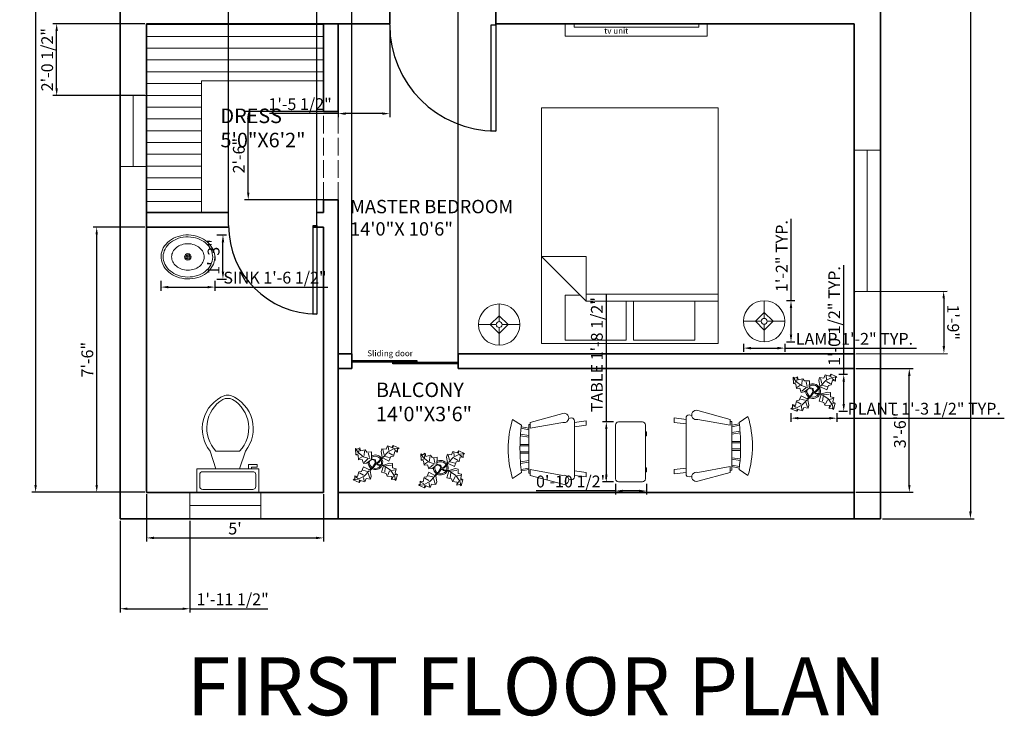
# Model space of a CAD drawing. Units: inches. Extents: x 2170 to 3011, y 1733 to 2338.
# Tile 4 of 5: x 2677 to 3011, y 1737 to 1974. Entities that reach past the tile are written whole.
import ezdxf

# ---------------------------------------------------------------- set-up
doc = ezdxf.new("R2010")
doc.units = ezdxf.units.IN
doc.linetypes.add('ACAD_ISO02W100', pattern=[15, 12, -3])
for name, color, linetype, lineweight in [('A-AREA-IDEN', 4, 'Continuous', 18), ('A-FLOR-CASE', 20, 'Continuous', 20), ('A-FLOR-CASE-PATT', 252, 'Continuous', 13), ('A-FLOR-FIXT', 20, 'Continuous', 18), ('A-WALL', 7, 'Continuous', 35), ('A-WALL-OVHD', 7, 'ACAD_ISO02W100', 18), ('dim', 11, 'Continuous', 18), ('door', 6, 'Continuous', 25), ('furnitures', 20, 'Continuous', 18), ('L-PLNT', 81, 'Continuous', 13), ('text', 4, 'Continuous', 18), ('window', 3, 'Continuous', 20)]:
    doc.layers.add(name, color=color, linetype=linetype, lineweight=lineweight)
doc.styles.get("Standard").update_dxf_attribs({"font": 'arial.ttf'})
doc.dimstyles.new('ISO-25', dxfattribs={"dimtxt": 4, "dimasz": 2.5, "dimexe": 1.25, "dimexo": 0.625, "dimtad": 1, "dimlunit": 3, "dimtxsty": 'Standard', "dimcen": 2.5, "dimadec": 0, "dimazin": 0, "dimtfac": 1, "dimtmove": 0, "dimatfit": 3, "dimfxl": 1, "dimarcsym": 0})

# ---------------------------------------------------------------- blocks, each defined once
blk = doc.blocks.new('*D36')
at = {"layer": 'Defpoints', "color": 0, "transparency": 16777216}
for p in [(2719.6, 2293.31), (2681.96, 1813.31), (2719.6, 1813.31)]:
    blk.add_point(p, dxfattribs=at)
at = {"layer": 'dim', "color": 0, "lineweight": -2, "transparency": 16777216}
for p, q in [((2718.97, 2293.31), (2680.71, 2293.31)), ((2681.96, 2290.81), (2681.96, 1815.81)), ((2718.97, 1813.31), (2680.71, 1813.31))]:
    blk.add_line(p, q, dxfattribs=at)
at = {"layer": 'dim', "color": 0, "transparency": 16777216}
for points in [[(2681.54, 2290.81), (2682.37, 2290.81), (2681.96, 2293.31)], [(2681.54, 1815.81), (2682.37, 1815.81), (2681.96, 1813.31)]]:
    blk.add_solid(points, dxfattribs=at)
at = {"layer": 'dim', "color": 0, "transparency": 16777216, "insert": (2679.29, 2053.31), "char_height": 4, "attachment_point": 5, "rotation": 90}
blk.add_mtext("40'", dxfattribs=at)
blk = doc.blocks.new('*U37')
for p, q in [((-40, 0), (-40, 6)), ((0, 0), (0, 6))]:
    blk.add_line(p, q)
blk.add_lwpolyline([(0, 0), (0, -40), (-1.75, -40), (-1.75, 0)], close=True)
blk.add_arc((0, 0), 40, 180, 270)
blk = doc.blocks.new('Bed - Queen')
for p, q in [((0, -80.00003), (0, 0)), ((0, 0), (59.99999, 0)), ((59.99999, 0), (59.99999, -80.00003)), ((7.99999, -1.2), (28.79998, -1.2)), ((7.99999, -14.4), (7.99999, -1.2)), ((28.79998, -1.2), (28.79998, -14.4)), ((31.19999, -1.2), (51.99999, -1.2)), ((31.19999, -14.4), (31.19999, -1.2)), ((51.99999, -1.2), (51.99999, -16.4)), ((0, -14.4), (44.8, -14.4)), ((59.99999, -29.6), (44.8, -14.4)), ((44.8, -14.4), (44.8, -29.6)), ((51.99999, -16.4), (46.79936, -16.4)), ((44.8, -16.8), (0, -16.8)), ((44.8, -29.6), (59.99999, -29.6)), ((59.99999, -80.00003), (0, -80.00003))]:
    blk.add_line(p, q)
blk = doc.blocks.new('Lamp - Table')
for p, q in [((0, 7), (0, 1)), ((-1, 0), (-7, 0)), ((0, 3), (-3, 0)), ((-3, 0), (0, -3)), ((3, 0), (0, 3)), ((0, -3), (3, 0)), ((1, 0), (7, 0)), ((0, -1), (0, -7))]:
    blk.add_line(p, q)
for radius in [7, 1]:
    blk.add_circle((0, 0), radius)
blk = doc.blocks.new('Plant - Rubber or Philodendron')
for p, q in [((-16.2005, 11.4774), (-13.9899, 8.1064)), ((-16.2005, 11.4774), (-14.8639, 10.7964)), ((-16.0159, 6.3329), (-16.2005, 11.4774)), ((-14.8639, 10.7964), (-12.6195, 11.8975)), ((-13.9899, 8.1064), (-9.5434, 4.7185)), ((-13.3174, 8.325), (-13.0735, 11.0065)), ((-12.6195, 11.8975), (-12.1909, 9.4345)), ((-12.1909, 9.4345), (-8.3829, 10.3)), ((-8.8369, 9.409), (-9.0894, 5.6095)), ((-8.3829, 10.3), (-7.0549, 8.501)), ((-7.0549, 8.501), (-3.0284, 8.6941)), ((-3.0284, 8.6941), (-3.0709, 3.1041)), ((4.6914, 8.8812), (5.3859, 11.2828)), ((4.6914, 8.8812), (5.5014, 4.4831)), ((5.3859, 11.2828), (8.8871, 10.7908)), ((5.9878, 10.4842), (7.1971, 6.3869)), ((10.3916, 8.7942), (6.2847, 4.4028)), ((8.8871, 10.7908), (9.9809, 13.4933)), ((9.9809, 13.4933), (13.3837, 12.301)), ((15.3859, 11.3055), (10.3916, 8.7942)), ((10.5828, 12.6946), (10.8893, 9.7953)), ((13.3837, 12.301), (14.68, 13.9039)), ((14.5816, 13.2037), (14.3848, 11.8033)), ((14.68, 13.9039), (19.3848, 11.8146)), ((15.7909, 9.1065), (14.8995, 5.3044)), ((15.2875, 10.6053), (17.5907, 9.2105)), ((19.3848, 11.8146), (15.3859, 11.3055)), ((18.1925, 8.4119), (15.7909, 9.1065)), ((19.3848, 11.8146), (18.1868, 10.9119)), ((18.1868, 10.9119), (18.1925, 8.4119)), ((-14.0069, 5.8704), (-16.0159, 6.3329)), ((-15.3434, 6.5514), (-13.9984, 6.9884)), ((-13.5868, 2.2894), (-14.0069, 5.8704)), ((-10.6784, 2.491), (-13.5868, 2.2894)), ((-13.1329, 3.1804), (-10.6614, 4.727)), ((-9.5858, -0.8715), (-10.6784, 2.491)), ((-9.5434, 4.7185), (-4.1917, 2.9888)), ((-9.1318, 0.0195), (-5.9793, 2.9025)), ((-7.1228, -0.443), (-3.5248, 2.2131)), ((-4.8529, 4.012), (-5.7184, 7.82)), ((-3.5248, 2.2131), (-3.3011, 2.4355)), ((-3.3011, 2.4355), (-0.5306, 1.7947)), ((-3.0709, 3.1041), (0.0797, 2.3163)), ((-0.5306, 1.7947), (-0.2255, -0.5527)), ((-0.5306, 1.7947), (-0.5306, 1.7947)), ((0.0797, 2.3163), (0.4866, -0.031)), ((0.4866, -0.031), (2.1141, 0.2298)), ((2.1141, 0.2298), (5.4346, 3.9146)), ((6.1032, 3.6844), (2.8262, -0.031)), ((5.4346, 3.9146), (5.5014, 4.4831)), ((11.1089, 1.1958), (6.1032, 3.6844)), ((7.7005, 4.8881), (11.5025, 3.9967)), ((14.2977, 6.1031), (10.9934, 7.9956)), ((12.7005, 4.8994), (11.1089, 1.1958)), ((14.8995, 5.3044), (12.7005, 4.8994)), ((-14.4141, -11.4699), (-13.5228, -7.6679)), ((-13.5228, -7.6679), (-11.3237, -7.2629)), ((-11.3237, -7.2629), (-9.7321, -3.5593)), ((-6.3237, -7.2516), (-10.1257, -6.3602)), ((-9.7321, -3.5593), (-4.7264, -6.0479)), ((-7.1228, -0.443), (-9.5858, -0.8715)), ((-9.0148, -11.1577), (-4.9047, -6.8122)), ((-2.019, -3.6148), (-4.7264, -6.0479)), ((-4.1246, -6.8466), (-4.0579, -6.2781)), ((-3.3146, -11.2447), (-4.1246, -6.8466)), ((-4.0579, -6.2781), (-0.9375, -3.1608)), ((-2.019, -3.6148), (-0.2255, -0.5527)), ((-0.9375, -3.1608), (0.5883, -0.8135)), ((0.5883, -0.8135), (2.2447, -2.0916)), ((2.8262, -0.031), (1.3003, -0.5527)), ((1.3003, -0.5527), (2.4193, -1.4655)), ((2.2447, -2.0916), (6.7108, -2.6626)), ((2.4193, -1.4655), (6.895, -2.1175)), ((4.943, -7.9659), (6.7108, -2.6626)), ((8.8321, -9.0266), (4.943, -7.9659)), ((11.6605, -0.5413), (6.895, -2.1175)), ((12.3677, -6.1981), (7.219, -2.6772)), ((8.125, -4.0768), (7.7715, -7.9659)), ((8.3544, -2.7453), (13.1973, -2.1704)), ((10.2463, -10.4408), (11.6605, -6.9053)), ((11.6605, -0.5413), (14.1354, -0.8948)), ((15.5496, -10.7943), (12.3677, -6.1981)), ((16.2567, -5.8446), (13.4283, -6.5517)), ((14.1354, -0.8948), (14.1354, -4.4304)), ((14.1354, -4.4304), (16.9638, -5.1375)), ((16.9638, -5.1375), (16.2567, -8.673)), ((-18.008, -14.1781), (-16.8101, -13.2754)), ((-18.008, -14.1781), (-14.0091, -13.669)), ((-13.3032, -16.2674), (-18.008, -14.1781)), ((-16.8157, -10.7754), (-14.4141, -11.4699)), ((-16.8101, -13.2754), (-16.8157, -10.7754)), ((-13.9107, -12.9688), (-16.2139, -11.574)), ((-14.0091, -13.669), (-9.0148, -11.1577)), ((-12.0069, -14.6645), (-13.3032, -16.2674)), ((-13.2048, -15.5672), (-13.008, -14.1668)), ((-12.921, -8.4665), (-9.6166, -10.359)), ((-8.6042, -15.8568), (-12.0069, -14.6645)), ((-9.206, -15.0581), (-9.5126, -12.1588)), ((-7.5103, -13.1543), (-8.6042, -15.8568)), ((-4.0092, -13.6463), (-7.5103, -13.1543)), ((-4.611, -12.8477), (-5.8203, -8.7504)), ((-3.3146, -11.2447), (-4.0092, -13.6463)), ((9.5392, -11.1479), (8.8321, -9.0266)), ((13.4283, -11.5015), (9.5392, -11.1479)), ((13.0748, -13.9763), (13.4283, -11.5015)), ((15.5496, -13.6228), (13.0748, -13.9763)), ((14.8425, -10.7943), (13.7819, -13.2692)), ((16.6103, -14.6834), (15.5496, -10.7943)), ((16.6103, -14.6834), (15.5496, -13.6228)), ((17.3174, -9.7337), (15.9032, -9.7337)), ((16.2567, -8.673), (18.0245, -9.7337)), ((18.0245, -9.7337), (16.6103, -14.6834))]:
    blk.add_line(p, q)
for centre, radius, start, end in [((0.0308, 0.1664), 6, 178.6147, 235.1169), ((0.0308, 0.1664), 5, 168.1647, 238.6725), ((0, 0), 6.1275, 34.37569, 120.1028), ((-0.0601, -0.2075), 5.2461, 33.82192, 124.9414), ((-0.2664, 0.1682), 5.2775, 338.4094, 20.03007), ((-0.098, 0.1364), 6.1288, 341.2017, 26.09184), ((-0.0234, 0.3825), 6.1492, 242.5812, 331.2714), ((-0.1102, 0.4886), 5.2883, 247.3711, 327.472)]:
    blk.add_arc(centre, radius, start, end)
blk = doc.blocks.new('Chair - Rocking')
for p, q in [((-8, -4.5), (-10, -1.5)), ((8, -4.5), (10, -1.5)), ((-7.5, -4.5), (-7, -7)), ((-6.5, -7), (-7.02225, -4.43)), ((-4.5, -7), (-4.96674, -4.19951)), ((-4, -7), (-4.40532, -4.16272)), ((-1.5, -4.05012), (-1.5, -7)), ((-1, -7), (-1, -4.05012)), ((1, -7), (1, -4.04655)), ((1.5, -4.05012), (1.5, -7)), ((4, -7), (4.40187, -4.18694)), ((4.5, -7), (4.96761, -4.19437)), ((6.5, -7), (7, -4.4057)), ((7.5, -4.5), (7, -7)), ((-9, -7.5), (-12, -18.49999)), ((-7, -7.5), (-9, -7.5)), ((-9, -18.49999), (-7, -7.5)), ((-8.23428, -6.99939), (-8.3093, -7.47958)), ((-8.23041, -7), (8.23915, -7)), ((7, -7.5), (9, -7.5)), ((9, -18.49999), (7, -7.5)), ((8.31071, -7.48854), (8.23449, -7.00073)), ((9, -7.5), (12, -18.49999)), ((-10.36644, -20.64523), (-10.5, -21.49999)), ((-9, -22.49999), (-9.5, -26.49999)), ((0, -22.49999), (-9.5, -22.49999)), ((-8, -26.49999), (-7.5, -22.49999)), ((0, -22.49999), (9.5, -22.49999)), ((8, -26.49999), (7.5, -22.49999)), ((9, -22.49999), (9.5, -26.49999)), ((10.5, -21.49999), (10.3575, -20.58798)), ((-9.5, -26.49999), (-8, -26.49999)), ((9.5, -26.49999), (8, -26.49999))]:
    blk.add_line(p, q)
for centre, radius, start, end in [((0, -34.08333), 34.08333, 72.93847, 107.0615), ((0, -68.25004), 64.25, 93.92211, 97.15267), ((0, -68.25004), 64.25, 82.84733, 93.92211), ((-10.5, -18.99999), 1.58114, 161.5651, 18.43495), ((10.5, -18.99999), 1.58114, 161.5651, 18.43495), ((-9.5, -21.49999), 1, 180, 270), ((9.5, -21.49999), 1, 270, 0)]:
    blk.add_arc(centre, radius, start, end)
blk = doc.blocks.new('Desk - 30 x 60 in.')
for p, q in [((-26.999995, 0), (26.999995, 0)), ((-29.999995, -27), (-29.999995, -3)), ((29.999995, -3), (29.999995, -27)), ((26.999995, -30), (-26.999995, -30)), ((-20.000005, -30), (-20.000005, -31)), ((-20.000005, -31), (-16.000005, -31)), ((-16.000005, -31), (-16.000005, -30)), ((15.999995, -31), (15.999995, -30)), ((19.999995, -31), (15.999995, -31)), ((19.999995, -30), (19.999995, -31))]:
    blk.add_line(p, q)
for centre, start, end in [((-26.499995, -3.5), 98.1301, 171.8699), ((26.499995, -3.5), 8.130102, 81.8699), ((-26.499995, -26.5), 188.1301, 261.8699), ((26.499995, -26.5), 278.1301, 351.8699)]:
    blk.add_arc(centre, 3.535534, start, end)
blk = doc.blocks.new('Toilet - top')
for p, q in [((9.5, -6), (9.5, -2)), ((-10, -8.5), (-8, -8.5)), ((-10, -9.5), (-10, -8.5)), ((-7, -9.5), (-10, -9.5)), ((-8, -8.5), (-8, -8)), ((-7, -8), (-7, -9.5)), ((-4, -8), (-6, -14)), ((4, -8), (6, -14)), ((4, -14), (-4, -14))]:
    blk.add_line(p, q)
blk.add_lwpolyline([(10.5, -8), (10.5, 0), (-10.5, 0), (-10.5, -8)], close=True)
for points in [[(-9.5, -2), (-9.5, -6)], [(8.5, -1), (-8.5, -1)], [(-8.5, -7), (8.5, -7)]]:
    blk.add_lwpolyline(points)
for centre, radius, start, end in [((-8.62, -1.88), 0.884, 81.8699, 188.1301), ((8.62, -1.88), 0.884, 351.8699, 98.1301), ((-8.62, -6.12), 0.884, 171.8699, 278.1301), ((8.62, -6.12), 0.884, 261.8699, 8.1301), ((3.52, -21.58), 12.17, 141.4691, 247.9714), ((4.2, -21.82), 11.33, 136.3677, 238.9468), ((-3.52, -21.58), 12.17, 292.0284, 38.5307), ((-4.2, -21.82), 11.33, 301.053, 43.6321), ((0, -27.88), 4, 245.7318, 294.2682), ((0, -29), 4, 254.8605, 285.1395)]:
    blk.add_arc(centre, radius, start, end)
blk = doc.blocks.new('Sink - Oval top')
for p, q in [((-1, 0), (1, 0)), ((0, 1), (0, -1))]:
    blk.add_line(p, q)
for points in [[(-12.23, 0.39, 0.117634), (-11.46, -3.36, 0.104469), (-8.88, -6.8, 0.090016), (-5.08, -9.07, 0.08192), (-0.32, -10.02, 0.08192), (4.49, -9.38, 0.090016), (8.42, -7.36, 0.104469), (11.22, -4.09, 0.117634), (12.23, -0.39, 0.117634), (11.46, 3.36, 0.104469), (8.88, 6.8, 0.090016), (5.08, 9.07, 0.08192), (0.32, 10.02, 0.08192), (-4.49, 9.38, 0.090016), (-8.42, 7.36, 0.104469), (-11.22, 4.09, 0.117634)], [(-11.29, 0.16, 0.118622), (-10.52, -3.25, 0.104678), (-8.07, -6.36, 0.089562), (-4.54, -8.37, 0.081185), (-0.13, -9.15, 0.081185), (4.3, -8.49, 0.089562), (7.89, -6.58, 0.104678), (10.42, -3.55, 0.118622), (11.29, -0.16, 0.118622), (10.52, 3.25, 0.104678), (8.07, 6.36, 0.089562), (4.54, 8.37, 0.081185), (0.13, 9.15, 0.081185), (-4.3, 8.49, 0.089562), (-7.89, 6.58, 0.104678), (-10.42, 3.55, 0.118622)], [(-7.42, 0.08, 0.118283), (-6.91, -2.17, 0.104607), (-5.29, -4.21, 0.089718), (-2.97, -5.53, 0.081436), (-0.07, -6.04, 0.081436), (2.84, -5.59, 0.089718), (5.2, -4.33, 0.104607), (6.86, -2.32, 0.118283), (7.42, -0.08, 0.118283), (6.91, 2.17, 0.104607), (5.29, 4.21, 0.089718), (2.97, 5.53, 0.081436), (0.07, 6.04, 0.081436), (-2.84, 5.59, 0.089718), (-5.2, 4.33, 0.104607), (-6.86, 2.32, 0.118283)]]:
    blk.add_lwpolyline(points, format="xyb", close=True)
for radius in [1.5, 1]:
    blk.add_circle((0, 0), radius)
blk = doc.blocks.new('*D38')
at = {"layer": 'Defpoints', "color": 0, "transparency": 16777216}
for p in [(2719.6, 1813.31), (2779.6, 1813.31), (2779.6, 1797.84)]:
    blk.add_point(p, dxfattribs=at)
at = {"layer": 'dim', "color": 0, "lineweight": -2, "transparency": 16777216}
for p, q in [((2719.6, 1812.68), (2719.6, 1796.59)), ((2779.6, 1812.68), (2779.6, 1796.59)), ((2722.1, 1797.84), (2777.1, 1797.84))]:
    blk.add_line(p, q, dxfattribs=at)
at = {"layer": 'dim', "color": 0, "transparency": 16777216}
for points in [[(2722.1, 1798.25), (2722.1, 1797.42), (2719.6, 1797.84)], [(2777.1, 1798.25), (2777.1, 1797.42), (2779.6, 1797.84)]]:
    blk.add_solid(points, dxfattribs=at)
at = {"layer": 'dim', "color": 0, "transparency": 16777216, "insert": (2749.6, 1800.49), "char_height": 4, "attachment_point": 5}
blk.add_mtext("5'", dxfattribs=at)
blk = doc.blocks.new('*D39')
at = {"layer": 'Defpoints', "color": 0, "transparency": 16777216}
for p in [(2702.69, 1903.31), (2719.6, 1903.31), (2719.6, 1813.31)]:
    blk.add_point(p, dxfattribs=at)
at = {"layer": 'dim', "color": 0, "lineweight": -2, "transparency": 16777216}
for p, q in [((2718.97, 1903.31), (2701.44, 1903.31)), ((2702.69, 1815.81), (2702.69, 1900.81)), ((2718.97, 1813.31), (2701.44, 1813.31))]:
    blk.add_line(p, q, dxfattribs=at)
at = {"layer": 'dim', "color": 0, "transparency": 16777216}
for points in [[(2702.27, 1900.81), (2703.1, 1900.81), (2702.69, 1903.31)], [(2702.27, 1815.81), (2703.1, 1815.81), (2702.69, 1813.31)]]:
    blk.add_solid(points, dxfattribs=at)
at = {"layer": 'dim', "color": 0, "transparency": 16777216, "insert": (2700.02, 1858.31), "char_height": 4, "attachment_point": 5, "rotation": 90}
blk.add_mtext('7\'-6"', dxfattribs=at)
blk = doc.blocks.new('*D40')
at = {"layer": 'Defpoints', "color": 0, "transparency": 16777216}
for p in [(2959.6, 1855.31), (2978.37, 1855.31), (2959.6, 1813.31)]:
    blk.add_point(p, dxfattribs=at)
at = {"layer": 'dim', "color": 0, "lineweight": -2, "transparency": 16777216}
for p, q in [((2960.22, 1855.31), (2979.62, 1855.31)), ((2978.37, 1815.81), (2978.37, 1852.81)), ((2960.22, 1813.31), (2979.62, 1813.31))]:
    blk.add_line(p, q, dxfattribs=at)
at = {"layer": 'dim', "color": 0, "transparency": 16777216}
for points in [[(2977.95, 1852.81), (2978.78, 1852.81), (2978.37, 1855.31)], [(2977.95, 1815.81), (2978.78, 1815.81), (2978.37, 1813.31)]]:
    blk.add_solid(points, dxfattribs=at)
at = {"layer": 'dim', "color": 0, "transparency": 16777216, "insert": (2975.7, 1834.31), "char_height": 4, "attachment_point": 5, "rotation": 90}
blk.add_mtext('3\'-6"', dxfattribs=at)
blk = doc.blocks.new('WINDOW-48x9')
blk.add_line((4.5, 48), (4.5, 0))
blk.add_lwpolyline([(0, 48), (9, 48), (9, 0), (0, 0)], close=True)
blk = doc.blocks.new('WINDOW-24x9')
blk.add_line((4.5, 24), (4.5, 0))
blk.add_lwpolyline([(0, 24), (9, 24), (9, 0), (0, 0)], close=True)
blk = doc.blocks.new('*D50')
at = {"layer": 'Defpoints', "color": 0, "transparency": 16777216}
for p in [(2922.13, 1864.34), (2936.13, 1864.34), (2936.13, 1862.24)]:
    blk.add_point(p, dxfattribs=at)
at = {"layer": 'dim', "color": 0, "lineweight": -2, "transparency": 16777216}
for p, q in [((2922.13, 1863.71), (2922.13, 1860.99)), ((2924.63, 1862.24), (2933.63, 1862.24)), ((2936.13, 1863.71), (2936.13, 1860.99)), ((2936.13, 1862.24), (2980.85, 1862.24))]:
    blk.add_line(p, q, dxfattribs=at)
at = {"layer": 'dim', "color": 0, "transparency": 16777216}
for points in [[(2924.63, 1862.66), (2924.63, 1861.82), (2922.13, 1862.24)], [(2933.63, 1862.66), (2933.63, 1861.82), (2936.13, 1862.24)]]:
    blk.add_solid(points, dxfattribs=at)
at = {"layer": 'dim', "color": 0, "transparency": 16777216, "insert": (2959.74, 1864.87), "char_height": 4, "attachment_point": 5}
blk.add_mtext('LAMP 1\'-2" TYP.', dxfattribs=at)
blk = doc.blocks.new('*D51')
at = {"layer": 'Defpoints', "color": 0, "transparency": 16777216}
for p in [(2936.13, 1878.34), (2938.23, 1878.34), (2936.13, 1864.34)]:
    blk.add_point(p, dxfattribs=at)
at = {"layer": 'dim', "color": 0, "lineweight": -2, "transparency": 16777216}
for p, q in [((2938.23, 1878.34), (2938.23, 1906.09)), ((2936.75, 1878.34), (2939.48, 1878.34)), ((2938.23, 1866.84), (2938.23, 1875.84)), ((2936.75, 1864.34), (2939.48, 1864.34))]:
    blk.add_line(p, q, dxfattribs=at)
at = {"layer": 'dim', "color": 0, "transparency": 16777216}
for points in [[(2937.81, 1875.84), (2938.65, 1875.84), (2938.23, 1878.34)], [(2937.81, 1866.84), (2938.65, 1866.84), (2938.23, 1864.34)]]:
    blk.add_solid(points, dxfattribs=at)
at = {"layer": 'dim', "color": 0, "transparency": 16777216, "insert": (2935.6, 1893.47), "char_height": 4, "attachment_point": 5, "rotation": 90}
blk.add_mtext('1\'-2" TYP.', dxfattribs=at)
blk = doc.blocks.new('*D52')
at = {"layer": 'Defpoints', "color": 0, "transparency": 16777216}
for p in [(2938.21, 1840.8), (2953.77, 1840.8), (2953.77, 1838.47)]:
    blk.add_point(p, dxfattribs=at)
at = {"layer": 'dim', "color": 0, "lineweight": -2, "transparency": 16777216}
for p, q in [((2938.21, 1840.17), (2938.21, 1837.22)), ((2940.71, 1838.47), (2951.27, 1838.47)), ((2953.77, 1840.17), (2953.77, 1837.22)), ((2953.77, 1838.47), (3010.59, 1838.47))]:
    blk.add_line(p, q, dxfattribs=at)
at = {"layer": 'dim', "color": 0, "transparency": 16777216}
for points in [[(2940.71, 1838.88), (2940.71, 1838.05), (2938.21, 1838.47)], [(2951.27, 1838.88), (2951.27, 1838.05), (2953.77, 1838.47)]]:
    blk.add_solid(points, dxfattribs=at)
at = {"layer": 'dim', "color": 0, "transparency": 16777216, "insert": (2983.43, 1841.16), "char_height": 4, "attachment_point": 5}
blk.add_mtext('PLANT 1\'-3 1/2" TYP.', dxfattribs=at)
blk = doc.blocks.new('*D53')
at = {"layer": 'Defpoints', "color": 0, "transparency": 16777216}
for p in [(2953.77, 1853.35), (2956.11, 1853.35), (2953.77, 1840.8)]:
    blk.add_point(p, dxfattribs=at)
at = {"layer": 'dim', "color": 0, "lineweight": -2, "transparency": 16777216}
for p, q in [((2956.11, 1853.35), (2956.11, 1890.43)), ((2954.4, 1853.35), (2957.36, 1853.35)), ((2956.11, 1843.3), (2956.11, 1850.85)), ((2954.4, 1840.8), (2957.36, 1840.8))]:
    blk.add_line(p, q, dxfattribs=at)
at = {"layer": 'dim', "color": 0, "transparency": 16777216}
for points in [[(2955.69, 1850.85), (2956.53, 1850.85), (2956.11, 1853.35)], [(2955.69, 1843.3), (2956.53, 1843.3), (2956.11, 1840.8)]]:
    blk.add_solid(points, dxfattribs=at)
at = {"layer": 'dim', "color": 0, "transparency": 16777216, "insert": (2953.42, 1873.14), "char_height": 4, "attachment_point": 5, "rotation": 90}
blk.add_mtext('1\'-0 1/2" TYP.', dxfattribs=at)
blk = doc.blocks.new('*D58')
at = {"layer": 'Defpoints', "color": 0, "transparency": 16777216}
for p in [(2724.5, 1885.68), (2742.78, 1885.68), (2742.78, 1882.94)]:
    blk.add_point(p, dxfattribs=at)
at = {"layer": 'dim', "color": 0, "lineweight": -2, "transparency": 16777216}
for p, q in [((2724.5, 1885.05), (2724.5, 1881.69)), ((2742.78, 1885.05), (2742.78, 1881.69)), ((2727, 1882.94), (2740.28, 1882.94)), ((2742.78, 1882.94), (2781.06, 1882.94))]:
    blk.add_line(p, q, dxfattribs=at)
at = {"layer": 'dim', "color": 0, "transparency": 16777216}
for points in [[(2727, 1883.35), (2727, 1882.52), (2724.5, 1882.94)], [(2740.28, 1883.35), (2740.28, 1882.52), (2742.78, 1882.94)]]:
    blk.add_solid(points, dxfattribs=at)
at = {"layer": 'dim', "color": 0, "transparency": 16777216, "insert": (2763.17, 1885.63), "char_height": 4, "attachment_point": 5}
blk.add_mtext('SINK 1\'-6 1/2"', dxfattribs=at)
blk = doc.blocks.new('*D59')
at = {"layer": 'Defpoints', "color": 0, "transparency": 16777216}
for p in [(2742.78, 1900.67), (2745.52, 1900.67), (2742.78, 1885.68)]:
    blk.add_point(p, dxfattribs=at)
at = {"layer": 'dim', "color": 0, "lineweight": -2, "transparency": 16777216}
for p, q in [((2743.4, 1900.67), (2746.77, 1900.67)), ((2745.52, 1888.18), (2745.52, 1898.17)), ((2743.4, 1885.68), (2746.77, 1885.68))]:
    blk.add_line(p, q, dxfattribs=at)
at = {"layer": 'dim', "color": 0, "transparency": 16777216}
for points in [[(2745.1, 1898.17), (2745.94, 1898.17), (2745.52, 1900.67)], [(2745.1, 1888.18), (2745.94, 1888.18), (2745.52, 1885.68)]]:
    blk.add_solid(points, dxfattribs=at)
at = {"layer": 'dim', "color": 0, "transparency": 16777216, "insert": (2742.85, 1893.17), "char_height": 4, "attachment_point": 5, "rotation": 90}
blk.add_mtext('1\'-3"', dxfattribs=at)
blk = doc.blocks.new('*D64')
at = {"layer": 'Defpoints', "color": 0, "transparency": 16777216}
for p in [(2875.58, 1837.25), (2878.64, 1837.25), (2878.64, 1816.83)]:
    blk.add_point(p, dxfattribs=at)
at = {"layer": 'dim', "color": 0, "lineweight": -2, "transparency": 16777216}
for p, q in [((2875.58, 1837.25), (2875.58, 1880.31)), ((2878.01, 1837.25), (2874.33, 1837.25)), ((2875.58, 1819.33), (2875.58, 1834.75)), ((2878.01, 1816.83), (2874.33, 1816.83))]:
    blk.add_line(p, q, dxfattribs=at)
at = {"layer": 'dim', "color": 0, "transparency": 16777216}
for points in [[(2875.16, 1834.75), (2875.99, 1834.75), (2875.58, 1837.25)], [(2875.16, 1819.33), (2875.99, 1819.33), (2875.58, 1816.83)]]:
    blk.add_solid(points, dxfattribs=at)
at = {"layer": 'dim', "color": 0, "transparency": 16777216, "insert": (2872.88, 1860.03), "char_height": 4, "attachment_point": 5, "rotation": 90}
blk.add_mtext('TABLE 1\'-8 1/2"', dxfattribs=at)
blk = doc.blocks.new('*D65')
at = {"layer": 'Defpoints', "color": 0, "transparency": 16777216}
for p in [(2878.64, 1816.83), (2889.19, 1816.83), (2878.64, 1813.77)]:
    blk.add_point(p, dxfattribs=at)
at = {"layer": 'dim', "color": 0, "lineweight": -2, "transparency": 16777216}
for p, q in [((2878.64, 1816.21), (2878.64, 1812.52)), ((2889.19, 1816.21), (2889.19, 1812.52)), ((2878.64, 1813.77), (2851.83, 1813.77)), ((2886.69, 1813.77), (2881.14, 1813.77))]:
    blk.add_line(p, q, dxfattribs=at)
at = {"layer": 'dim', "color": 0, "transparency": 16777216}
for points in [[(2881.14, 1814.19), (2881.14, 1813.36), (2878.64, 1813.77)], [(2886.69, 1814.19), (2886.69, 1813.36), (2889.19, 1813.77)]]:
    blk.add_solid(points, dxfattribs=at)
at = {"layer": 'dim', "color": 0, "transparency": 16777216, "insert": (2863.98, 1816.47), "char_height": 4, "attachment_point": 5}
blk.add_mtext('0\'-10 1/2"', dxfattribs=at)
blk = doc.blocks.new('*D94')
at = {"layer": 'Defpoints', "color": 0, "transparency": 16777216}
for p in [(2959.52, 1881.46), (2959.6, 1860.31), (2990.1, 1860.43)]:
    blk.add_point(p, dxfattribs=at)
at = {"layer": 'dim', "color": 0, "lineweight": -2, "transparency": 16777216}
for p, q in [((2960.14, 1881.46), (2991.26, 1881.59)), ((2990.02, 1879.08), (2990.09, 1862.93)), ((2960.22, 1860.31), (2991.35, 1860.43))]:
    blk.add_line(p, q, dxfattribs=at)
at = {"layer": 'dim', "color": 0, "transparency": 16777216}
for points in [[(2990.44, 1879.08), (2989.61, 1879.08), (2990.01, 1881.58)], [(2990.51, 1862.93), (2989.67, 1862.93), (2990.1, 1860.43)]]:
    blk.add_solid(points, dxfattribs=at)
at = {"layer": 'dim', "color": 0, "transparency": 16777216, "insert": (2992.72, 1871.02), "char_height": 4, "attachment_point": 5, "rotation": 270.2297}
blk.add_mtext('1\'-9"', dxfattribs=at)
blk = doc.blocks.new('*D95')
at = {"layer": 'Defpoints', "color": 0, "transparency": 16777216}
for p in [(2689.1, 1972.31), (2719.6, 1972.31), (2719.6, 1947.91)]:
    blk.add_point(p, dxfattribs=at)
at = {"layer": 'dim', "color": 0, "lineweight": -2, "transparency": 16777216}
for p, q in [((2718.97, 1972.31), (2687.85, 1972.31)), ((2689.1, 1950.41), (2689.1, 1969.81)), ((2718.97, 1947.91), (2687.85, 1947.91))]:
    blk.add_line(p, q, dxfattribs=at)
at = {"layer": 'dim', "color": 0, "transparency": 16777216}
for points in [[(2688.68, 1969.81), (2689.52, 1969.81), (2689.1, 1972.31)], [(2688.68, 1950.41), (2689.52, 1950.41), (2689.1, 1947.91)]]:
    blk.add_solid(points, dxfattribs=at)
at = {"layer": 'dim', "color": 0, "transparency": 16777216, "insert": (2686.41, 1960.11), "char_height": 4, "attachment_point": 5, "rotation": 90}
blk.add_mtext('2\'-0 1/2"', dxfattribs=at)
blk = doc.blocks.new('*D96')
at = {"layer": 'Defpoints', "color": 0, "transparency": 16777216}
for p in [(2710.6, 1804.31), (2734.32, 1804.31), (2734.32, 1773.81)]:
    blk.add_point(p, dxfattribs=at)
at = {"layer": 'dim', "color": 0, "lineweight": -2, "transparency": 16777216}
for p, q in [((2710.6, 1803.68), (2710.6, 1772.56)), ((2734.32, 1803.68), (2734.32, 1772.56)), ((2713.1, 1773.81), (2731.82, 1773.81)), ((2734.32, 1773.81), (2760.76, 1773.81))]:
    blk.add_line(p, q, dxfattribs=at)
at = {"layer": 'dim', "color": 0, "transparency": 16777216}
for points in [[(2713.1, 1774.22), (2713.1, 1773.39), (2710.6, 1773.81)], [(2731.82, 1774.22), (2731.82, 1773.39), (2734.32, 1773.81)]]:
    blk.add_solid(points, dxfattribs=at)
at = {"layer": 'dim', "color": 0, "transparency": 16777216, "insert": (2748.79, 1776.5), "char_height": 4, "attachment_point": 5}
blk.add_mtext('1\'-11 1/2"', dxfattribs=at)
blk = doc.blocks.new('*D97')
at = {"layer": 'Defpoints', "color": 0, "transparency": 16777216}
for p in [(2825.28, 2332.81), (2789.28, 1855.31), (2825.28, 1855.31)]:
    blk.add_point(p, dxfattribs=at)
at = {"layer": 'dim', "color": 0, "lineweight": -2, "transparency": 16777216}
for p, q in [((2789.28, 1855.93), (2789.28, 2334.06)), ((2791.78, 2332.81), (2822.78, 2332.81)), ((2825.28, 1855.93), (2825.28, 2334.06))]:
    blk.add_line(p, q, dxfattribs=at)
at = {"layer": 'dim', "color": 0, "transparency": 16777216}
for points in [[(2791.78, 2333.22), (2791.78, 2332.39), (2789.28, 2332.81)], [(2822.78, 2333.22), (2822.78, 2332.39), (2825.28, 2332.81)]]:
    blk.add_solid(points, dxfattribs=at)
at = {"layer": 'dim', "color": 0, "transparency": 16777216, "insert": (2807.28, 2335.48), "char_height": 4, "attachment_point": 5}
blk.add_mtext('3\'-0"', dxfattribs=at)
blk = doc.blocks.new('*D98')
at = {"layer": 'Defpoints', "color": 0, "transparency": 16777216}
for p in [(2777.42, 2332.81), (2747.42, 1903.31), (2777.42, 1903.81)]:
    blk.add_point(p, dxfattribs=at)
at = {"layer": 'dim', "color": 0, "lineweight": -2, "transparency": 16777216}
for p, q in [((2747.42, 1903.93), (2747.42, 2334.06)), ((2749.92, 2332.81), (2774.92, 2332.81)), ((2777.42, 1904.43), (2777.42, 2334.06))]:
    blk.add_line(p, q, dxfattribs=at)
at = {"layer": 'dim', "color": 0, "transparency": 16777216}
for points in [[(2749.92, 2333.22), (2749.92, 2332.39), (2747.42, 2332.81)], [(2774.92, 2333.22), (2774.92, 2332.39), (2777.42, 2332.81)]]:
    blk.add_solid(points, dxfattribs=at)
at = {"layer": 'dim', "color": 0, "transparency": 16777216, "insert": (2762.42, 2335.47), "char_height": 4, "attachment_point": 5}
blk.add_mtext('2\'-6"', dxfattribs=at)
blk = doc.blocks.new('*D99')
at = {"layer": 'Defpoints', "color": 0, "transparency": 16777216}
for p in [(2754.1, 1942.54), (2784.6, 1942.54), (2784.6, 1912.54)]:
    blk.add_point(p, dxfattribs=at)
at = {"layer": 'dim', "color": 0, "lineweight": -2, "transparency": 16777216}
for p, q in [((2783.97, 1942.54), (2752.85, 1942.54)), ((2754.1, 1915.04), (2754.1, 1940.04)), ((2783.97, 1912.54), (2752.85, 1912.54))]:
    blk.add_line(p, q, dxfattribs=at)
at = {"layer": 'dim', "color": 0, "transparency": 16777216}
for points in [[(2753.68, 1940.04), (2754.52, 1940.04), (2754.1, 1942.54)], [(2753.68, 1915.04), (2754.52, 1915.04), (2754.1, 1912.54)]]:
    blk.add_solid(points, dxfattribs=at)
at = {"layer": 'dim', "color": 0, "transparency": 16777216, "insert": (2751.43, 1927.54), "char_height": 4, "attachment_point": 5, "rotation": 90}
blk.add_mtext('2\'-6"', dxfattribs=at)
blk = doc.blocks.new('*D101')
at = {"layer": 'Defpoints', "color": 0, "transparency": 16777216}
for p in [(2968.6, 2302.31), (2968.6, 1804.31), (2999.1, 1804.31)]:
    blk.add_point(p, dxfattribs=at)
at = {"layer": 'dim', "color": 0, "lineweight": -2, "transparency": 16777216}
for p, q in [((2969.22, 2302.31), (3000.35, 2302.31)), ((2999.1, 2299.81), (2999.1, 1806.81)), ((2969.22, 1804.31), (3000.35, 1804.31))]:
    blk.add_line(p, q, dxfattribs=at)
at = {"layer": 'dim', "color": 0, "transparency": 16777216}
for points in [[(2998.68, 2299.81), (2999.52, 2299.81), (2999.1, 2302.31)], [(2998.68, 1806.81), (2999.52, 1806.81), (2999.1, 1804.31)]]:
    blk.add_solid(points, dxfattribs=at)
at = {"layer": 'dim', "color": 0, "transparency": 16777216, "insert": (2996.43, 2053.31), "char_height": 4, "attachment_point": 5, "rotation": 90}
blk.add_mtext('41\'-6"', dxfattribs=at)
blk = doc.blocks.new('*D106')
at = {"layer": 'Defpoints', "color": 0, "transparency": 16777216}
for p in [(2784.6, 1972.31), (2802.09, 1972.31), (2784.6, 1941.81)]:
    blk.add_point(p, dxfattribs=at)
at = {"layer": 'dim', "color": 0, "lineweight": -2, "transparency": 16777216}
for p, q in [((2784.6, 1971.68), (2784.6, 1940.56)), ((2802.09, 1971.68), (2802.09, 1940.56)), ((2784.6, 1941.81), (2761.27, 1941.81)), ((2799.59, 1941.81), (2787.1, 1941.81))]:
    blk.add_line(p, q, dxfattribs=at)
at = {"layer": 'dim', "color": 0, "transparency": 16777216}
for points in [[(2787.1, 1942.22), (2787.1, 1941.39), (2784.6, 1941.81)], [(2799.59, 1942.22), (2799.59, 1941.39), (2802.09, 1941.81)]]:
    blk.add_solid(points, dxfattribs=at)
at = {"layer": 'dim', "color": 0, "transparency": 16777216, "insert": (2771.69, 1944.5), "char_height": 4, "attachment_point": 5}
blk.add_mtext('1\'-5 1/2"', dxfattribs=at)

msp = doc.modelspace()

# ---------------------------------------------------------------- hatches: boundary and pattern name
at = {"layer": 'A-FLOR-CASE-PATT'}
h = msp.add_hatch(dxfattribs=at)
h.set_pattern_fill('ANSI31', color=256, scale=1.259843, angle=-45, style=0)
h.paths.add_polyline_path([(2719.6, 1908.306), (2738.263, 1908.306), (2738.263, 1952.886), (2779.6, 1952.886), (2779.6, 1972.306), (2719.6, 1972.306)])

# ---------------------------------------------------------------- linework, layer by layer
at = {"layer": 'A-FLOR-CASE'}
for p, q in [((2779.6, 1972.306), (2719.6, 1972.306)), ((2719.6, 1972.306), (2719.6, 1952.886)), ((2779.6, 1952.886), (2779.6, 1972.306)), ((2864.647, 1972.306), (2864.647, 1971.167)), ((2864.647, 1971.167), (2906.988, 1971.167)), ((2906.988, 1971.167), (2906.988, 1972.306)), ((2738.263, 1952.886), (2779.6, 1952.886))]:
    msp.add_line(p, q, dxfattribs=at)
msp.add_lwpolyline([(2738.263, 1952.886), (2738.263, 1908.306), (2719.6, 1908.306), (2719.6, 1972.306), (2738.263, 1972.306)], dxfattribs=at)
msp.add_lwpolyline([(2861.638, 1972.306), (2909.775, 1972.306), (2909.775, 1968.138), (2861.638, 1968.138)], close=True, dxfattribs=at)
at = {"layer": 'A-WALL'}
for p, q in [((2710.6, 1804.306), (2710.6, 2302.306)), ((2968.6, 1804.306), (2968.6, 2302.306)), ((2719.6, 1813.306), (2719.6, 1972.306)), ((2719.6, 1972.306), (2784.944, 1972.306)), ((2779.6, 1942.538), (2779.6, 1972.306)), ((2784.6, 1942.538), (2784.6, 1972.306)), ((2784.944, 1972.306), (2802.086, 1972.306)), ((2838.086, 1972.306), (2959.6, 1972.306)), ((2898.861, 1972.306), (2959.6, 1972.306)), ((2959.6, 1804.306), (2959.6, 1972.306)), ((2959.6, 1972.306), (2959.6, 1813.306)), ((2779.6, 1908.306), (2779.6, 1912.538)), ((2784.6, 1804.306), (2784.6, 1912.538)), ((2719.6, 1908.306), (2747.416, 1908.306)), ((2747.416, 1908.306), (2719.6, 1908.306)), ((2779.6, 1908.306), (2777.416, 1908.306)), ((2777.416, 1908.306), (2779.6, 1908.306)), ((2719.6, 1903.306), (2747.42, 1903.306)), ((2776.103, 1903.306), (2779.6, 1903.306)), ((2779.6, 1813.306), (2779.6, 1903.306)), ((2784.6, 1860.306), (2789.28, 1860.306)), ((2825.28, 1860.306), (2959.6, 1860.306)), ((2784.6, 1855.306), (2789.28, 1855.306)), ((2825.28, 1855.306), (2959.6, 1855.306)), ((2719.6, 1813.306), (2779.6, 1813.306)), ((2784.6, 1813.306), (2959.6, 1813.306)), ((2710.6, 1804.306), (2959.6, 1804.306)), ((2959.6, 1804.306), (2968.6, 1804.306))]:
    msp.add_line(p, q, dxfattribs=at)
for points in [[(2802.086, 1972.306), (2802.086, 1977.306)], [(2838.086, 1977.306), (2838.086, 1972.306)], [(2779.6, 1942.538), (2784.6, 1942.538)], [(2784.6, 1912.538), (2779.6, 1912.538)], [(2789.28, 1855.306), (2789.28, 1860.306)], [(2825.28, 1860.306), (2825.28, 1855.306)]]:
    msp.add_lwpolyline(points, dxfattribs=at)
at = {"layer": 'A-WALL-OVHD', "ltscale": 0.5}
for p, q in [((2779.6, 1912.538), (2779.6, 1942.538)), ((2784.6, 1912.538), (2784.6, 1942.538))]:
    msp.add_line(p, q, dxfattribs=at)
at = {"layer": 'door'}
for points in [[(2789.28, 1858.086), (2811.324, 1858.086), (2811.324, 1857.527), (2789.28, 1857.527)], [(2803.181, 1857.513), (2825.225, 1857.513), (2825.225, 1856.954), (2803.181, 1856.954)]]:
    msp.add_lwpolyline(points, close=True, dxfattribs=at)

# ---------------------------------------------------------------- block references
at = {"layer": 'A-FLOR-FIXT', "xscale": 0.7444317497520238, "yscale": 0.7444317497520238, "zscale": 0.7444317497520238}
msp.add_blockref('Sink - Oval top', (2733.641, 1893.172), dxfattribs=at)
at = {"layer": 'A-FLOR-FIXT', "rotation": 180.0000413745557}
msp.add_blockref('Toilet - top', (2747.151, 1813.306), dxfattribs=at)
at = {"layer": 'door'}
for p, xscale, yscale, zscale in [((2838.086, 1971.906), 0.9, 0.9, 0.9), ((2777.416, 1903.806), 0.75, 0.75, 0.75)]:
    msp.add_blockref('*U37', p, dxfattribs=dict(at, xscale=xscale, yscale=yscale, zscale=zscale))
at = {"layer": 'furnitures'}
for name, p, rotation in [('Bed - Queen', (2913.56, 1863.761), 180), ('Chair - Rocking', (2925.134, 1829.054), 270), ('Chair - Rocking', (2842.287, 1828.056), 89.99997727777031)]:
    msp.add_blockref(name, p, dxfattribs=dict(at, rotation=rotation))
for p in [(2929.13, 1871.339), (2839.223, 1870.221)]:
    msp.add_blockref('Lamp - Table', p, dxfattribs=at)
at = {"layer": 'furnitures', "xscale": 0.340298145602901, "yscale": 0.340298145602901, "zscale": 0.340298145602901, "rotation": 90}
msp.add_blockref('Desk - 30 x 60 in.', (2878.638, 1827.044), dxfattribs=at)
at = {"layer": 'L-PLNT', "xscale": 0.4161339456418365, "yscale": 0.4161339456418365, "zscale": 0.4161339456418365}
for p in [(2945.708, 1847.569), (2797.21, 1823.426), (2819.403, 1821.59)]:
    msp.add_blockref('Plant - Rubber or Philodendron', p, dxfattribs=at)
at = {"layer": 'window'}
for name, p in [('WINDOW-24x9', (2710.6, 1923.911)), ('WINDOW-48x9', (2959.515, 1881.46))]:
    msp.add_blockref(name, p, dxfattribs=at)
at = {"layer": 'window', "rotation": 89.9999999999977}
msp.add_blockref('WINDOW-24x9', (2758.325, 1804.306), dxfattribs=at)

# ---------------------------------------------------------------- texts
at = {"layer": 'A-AREA-IDEN', "attachment_point": 1}
for s, width, gutter_width, insert, char_height in [('DRESS\\P5\'0"X6\'2"', 48.71482, 12.3, (2744.685, 1943.506), 4.9201), ('MASTER BEDROOM\\P14\'0"X 10\'6"', 74.52558, 11.361, (2788.64, 1912.538), 4.54432), ('BALCONY\\P14\'0"X3\'6"', 48.71482, 12.3, (2797.441, 1850.551), 4.9201)]:
    msp.add_mtext_dynamic_manual_height_columns(s, width=width, gutter_width=gutter_width, heights=[0], dxfattribs=dict(at, insert=insert, char_height=char_height))
at = {"layer": 'text'}
msp.add_text('FIRST FLOOR PLAN', height=19.6749, dxfattribs=at).set_placement((2733.2, 1737.66))
at = {"layer": 'text', "char_height": 2, "attachment_point": 1}
for s, insert in [('{\\fArial|b1|i1|c0|p34;tv unit}', (2874.869, 1970.898)), ('{\\fArial|b1|i1|c0|p34;Sliding door}', (2794.484, 1861.48))]:
    msp.add_mtext_dynamic_manual_height_columns(s, width=48.71482, gutter_width=12.3, heights=[0], dxfattribs=dict(at, insert=insert))

# ---------------------------------------------------------------- dimensions: what is measured, and where the dimension line sits
at = {"layer": 'dim'}
for base, p1, p2, override, picture, middle in [((2777.416, 2332.806), (2747.42, 1903.306), (2777.416, 1903.806), {"dimdec": 1, "dimlfac": 1, "dimrnd": 0, "dimzin": 1, "dimdsep": 46, "dimlunit": 4, "dimfrac": 2}, '*D98', (2762.418, 2335.474)), ((2825.28, 2332.806), (2789.28, 1855.306), (2825.28, 1855.306), {"dimdec": 1, "dimlfac": 1, "dimrnd": 0, "dimzin": 1, "dimdsep": 46, "dimlunit": 4, "dimfrac": 2}, '*D97', (2807.28, 2335.475)), ((2779.6, 1797.836), (2719.6, 1813.306), (2779.6, 1813.306), {"dimclrd": 0, "dimclre": 0, "dimclrt": 0}, '*D38', (2749.6, 1800.495)), ((2734.325, 1773.806), (2710.6, 1804.306), (2734.325, 1804.306), {"dimdec": 1, "dimlfac": 1, "dimrnd": 0, "dimzin": 1, "dimdsep": 46, "dimlunit": 4, "dimfrac": 2}, '*D96', (2748.792, 1776.5))]:
    dim = msp.add_linear_dim(base=base, p1=p1, p2=p2, dimstyle='ISO-25', override=override, dxfattribs=at)
    dim.commit()
    dim.dimension.update_dxf_attribs({"geometry": picture, "text_midpoint": middle})
for base, p1, p2, angle, override, picture, middle in [((2999.1, 1804.306), (2968.6, 2302.306), (2968.6, 1804.306), 270, {"dimdec": 1, "dimlfac": 1, "dimrnd": 0, "dimzin": 1, "dimdsep": 46, "dimlunit": 4, "dimfrac": 2}, '*D101', (2996.433, 2053.306)), ((2681.955, 1813.306), (2719.6, 2293.306), (2719.6, 1813.306), 90, {"dimclrd": 0, "dimclre": 0, "dimclrt": 0}, '*D36', (2679.288, 2053.306)), ((2689.1, 1972.306), (2719.6, 1947.911), (2719.6, 1972.306), 90, {"dimdec": 1, "dimlfac": 1, "dimrnd": 0, "dimzin": 1, "dimdsep": 46, "dimlunit": 4, "dimfrac": 2}, '*D95', (2686.407, 1960.109)), ((2784.6, 1941.806), (2802.086, 1972.306), (2784.6, 1972.306), 180, {"dimdec": 1, "dimlfac": 1, "dimrnd": 0, "dimzin": 1, "dimdsep": 46, "dimlunit": 4, "dimfrac": 2}, '*D106', (2771.686, 1944.5)), ((2754.1, 1942.538), (2784.6, 1912.538), (2784.6, 1942.538), 90, {"dimdec": 1, "dimlfac": 1, "dimrnd": 0, "dimzin": 1, "dimdsep": 46, "dimlunit": 4, "dimfrac": 2}, '*D99', (2751.433, 1927.538)), ((2702.685, 1903.306), (2719.6, 1813.306), (2719.6, 1903.306), 90, {"dimclrd": 0, "dimclre": 0, "dimclrt": 0}, '*D39', (2700.018, 1858.306)), ((2745.52, 1900.667), (2742.779, 1885.677), (2742.779, 1900.667), 90, {"dimdec": 1, "dimlfac": 1, "dimrnd": 0, "dimzin": 1, "dimdsep": 46, "dimlunit": 4, "dimfrac": 2}, '*D59', (2742.852, 1893.172)), ((2990.1, 1860.429), (2959.515, 1881.46), (2959.6, 1860.306), 270.2297, {"dimdec": 1, "dimlfac": 1, "dimrnd": 0, "dimzin": 1, "dimdsep": 46, "dimlunit": 4, "dimfrac": 2}, '*D94', (2992.725, 1871.016)), ((2978.367, 1855.306), (2959.6, 1813.306), (2959.6, 1855.306), 90, {"dimclrd": 0, "dimclre": 0, "dimclrt": 0}, '*D40', (2975.698, 1834.306)), ((2878.638, 1813.772), (2889.187, 1816.835), (2878.638, 1816.835), 180, {"dimdec": 1, "dimlfac": 1, "dimrnd": 0, "dimzin": 1, "dimdsep": 46, "dimlunit": 4, "dimfrac": 2}, '*D65', (2863.982, 1816.465))]:
    dim = msp.add_linear_dim(base=base, p1=p1, p2=p2, angle=angle, dimstyle='ISO-25', override=override, dxfattribs=at)
    dim.commit()
    dim.dimension.update_dxf_attribs({"geometry": picture, "text_midpoint": middle})
for base, p1, p2, text, picture, middle in [((2938.23, 1878.339), (2936.13, 1864.339), (2936.13, 1878.339), '<> TYP.', '*D51', (2935.595, 1893.467)), ((2956.109, 1853.354), (2953.775, 1840.799), (2953.775, 1853.354), '<> TYP.', '*D53', (2953.416, 1873.142)), ((2875.575, 1837.253), (2878.638, 1816.835), (2878.638, 1837.253), 'TABLE <>', '*D64', (2872.882, 1860.032))]:
    dim = msp.add_linear_dim(base=base, p1=p1, p2=p2, angle=90, text=text, dimstyle='ISO-25', override={"dimdec": 1, "dimlfac": 1, "dimrnd": 0, "dimzin": 1, "dimdsep": 46, "dimlunit": 4, "dimfrac": 2}, dxfattribs=at)
    dim.commit()
    dim.dimension.update_dxf_attribs({"geometry": picture, "text_midpoint": middle})
for base, p1, p2, text, picture, middle in [((2742.779, 1882.936), (2724.503, 1885.677), (2742.779, 1885.677), 'SINK <>', '*D58', (2763.169, 1885.629)), ((2936.13, 1862.239), (2922.13, 1864.339), (2936.13, 1864.339), 'LAMP <> TYP.', '*D50', (2959.742, 1864.874)), ((2953.775, 1838.465), (2938.214, 1840.799), (2953.775, 1840.799), 'PLANT <> TYP.', '*D52', (2983.433, 1841.16))]:
    dim = msp.add_linear_dim(base=base, p1=p1, p2=p2, text=text, dimstyle='ISO-25', override={"dimdec": 1, "dimlfac": 1, "dimrnd": 0, "dimzin": 1, "dimdsep": 46, "dimlunit": 4, "dimfrac": 2}, dxfattribs=at)
    dim.commit()
    dim.dimension.update_dxf_attribs({"geometry": picture, "text_midpoint": middle})

doc.saveas('drawing.dxf')
